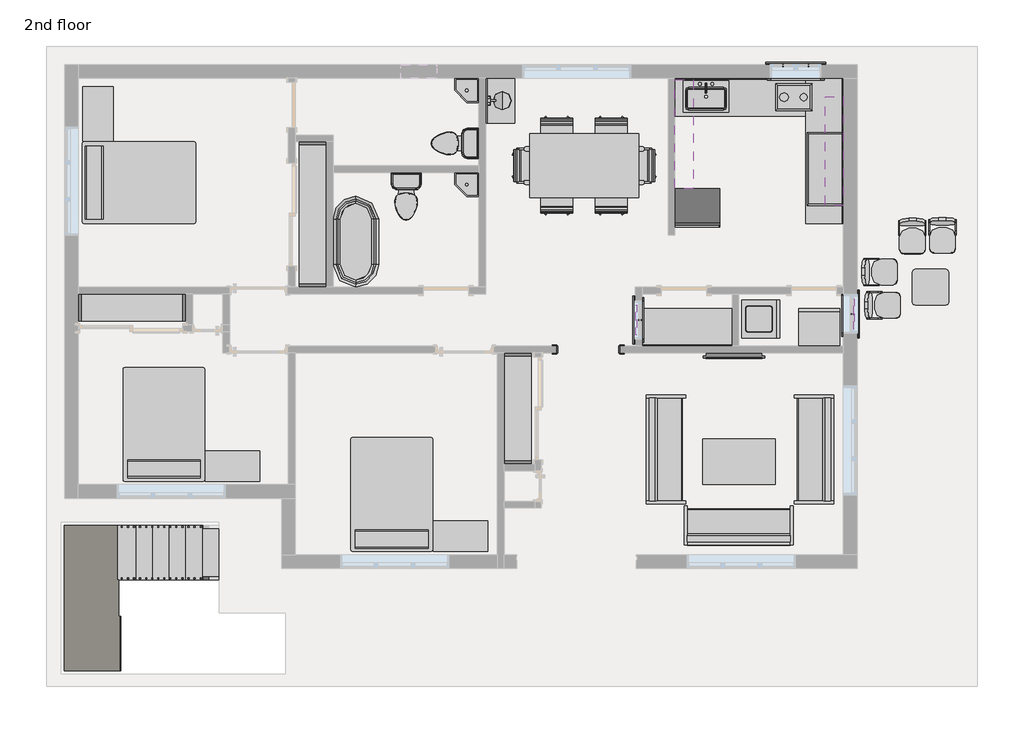
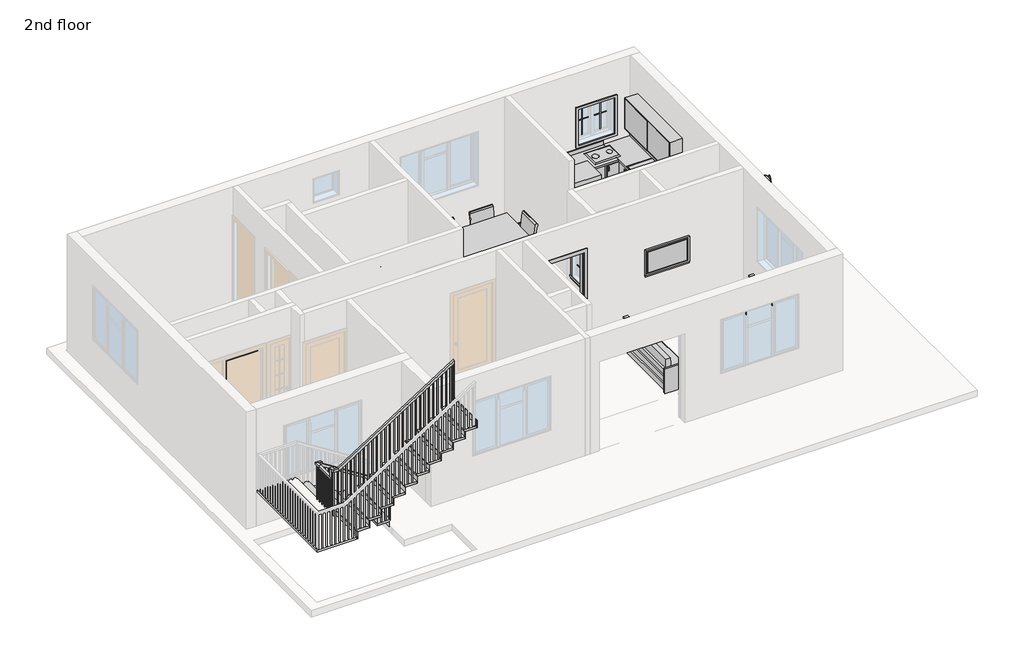
# One storey, part 4 of 4: 34 furniture elements, 17 proxies, 7 flow terminals, 2 stair flights, 1 railing, 1 slab.
"""IFC4 building model written with IfcOpenShell, lengths in millimetres."""

from ifc_helpers import new_model, si_unit, frame, origin, place, context, project, spatial, polyline, outline, extrude, faceted_brep, transform, mapped, element, save
from components import proxy_3c1fa1d0, proxy_97c73763, muntin_pattern_2x2_muntin_pattern_2x2_b3fe6957, muntin_pattern_2x2_muntin_pattern_2x2_3e0ecaf2, muntin_pattern_2x2_muntin_pattern_2x2_c35c595f, muntin_pattern_2x2_muntin_pattern_2x2_183aef24, proxy_bc9927fa, proxy_e6cf46b9, trim_window_exterior_flat_with_sill_41619996, trim_window_exterior_flat_with_sill_e38017c9, trim_window_exterior_flat_with_sill_5e960bf5, trim_window_interior_flat_picture_frame_51c85655, trim_window_interior_flat_picture_frame_d728ed12, trim_window_interior_flat_picture_frame_80babb00, proxy_1934c8a4, flow_terminal_15267b2a, flow_terminal_5b58e753, flow_terminal_4d548711, toilet_domestic_3d_toilet_domestic_3d_ba6479b0, toilet_domestic_3d_toilet_domestic_3d_30431060, flow_terminal_ce36f001, furniture_48488436, furniture_f87f75a4, furniture_97fe820d, furniture_52ef1662, furniture_6b884072, chair_task_chair_task_b7f3823b, chair_task_arms_chair_task_arms_fa5a08ef, furniture_deb1c5d1, furniture_9388d8e7, furniture_74614b7d, furniture_eb3a3c23, furniture_53a00f75, furniture_df918c0e, furniture_57be741f, furniture_57f9710a, furniture_acc2807d, furniture_65ba067b, furniture_5d68651d, furniture_b6aab1a0, furniture_1cc80a06, non_monolithic_landing_c00d822c, stair_flight_b9929406, stair_flight_87f1d909

model = new_model("IFC4")

# Units and contexts
model_context = context("Model", 3, world=origin())
ifc_project = project(units=[si_unit("LENGTHUNIT", "METRE", prefix="MILLI")], contexts=[model_context])

# Site, building, storey
site = spatial("IfcSite", under=ifc_project)
building = spatial("IfcBuilding", under=site)
storey = spatial("IfcBuildingStorey", under=building, Name="2nd floor", Elevation=7010.4)

# Proxies
placement = place(None, origin())
proxy_shape = proxy_3c1fa1d0(model_context)
element("IfcBuildingElementProxy", 1, Name="Cook Top-2 Unit : 12\" x 18\"", ObjectType="Cook Top-2 Unit : 12\" x 18\"", at=placement, inside=storey, context=model_context, shape_type="MappedRepresentation", body=[
    mapped(proxy_shape, transform((3099.7984427, 6060.3661978, 7010.4), x_axis=(0.0, 1.0, 0.0), y_axis=(-1.0, 0.0, 0.0), z_axis=(0.0, 0.0, 1.0))),
])
proxy_2_shape = proxy_97c73763(model_context)
element("IfcBuildingElementProxy", 2, Name="Dryer : 27\" x 25\" x 35\"", ObjectType="Dryer : 27\" x 25\" x 35\"", at=placement, inside=storey, context=model_context, shape_type="MappedRepresentation", body=[
    mapped(proxy_2_shape, transform((3116.0361908, 1961.105194, 7010.4), x_axis=(1.0, 0.0, 0.0), y_axis=(0.0, 1.0, 0.0), z_axis=(0.0, 0.0, 1.0))),
])
muntin_pattern_2x2_muntin_pattern_2x2_shape = muntin_pattern_2x2_muntin_pattern_2x2_b3fe6957(model_context)
element("IfcBuildingElementProxy", 3, Name="Muntin Pattern_2x2 : Muntin Pattern_2x2", ObjectType="Muntin Pattern_2x2 : Muntin Pattern_2x2", at=placement, inside=storey, context=model_context, shape_type="MappedRepresentation", body=[
    mapped(muntin_pattern_2x2_muntin_pattern_2x2_shape, transform((2887.0111471, 6673.1411978, 8172.45), x_axis=(1.0, 0.0, 0.0), y_axis=(0.0, 1.0, 0.0), z_axis=(0.0, 0.0, 1.0))),
])
muntin_pattern_2x2_muntin_pattern_2x2_2_shape = muntin_pattern_2x2_muntin_pattern_2x2_3e0ecaf2(model_context)
element("IfcBuildingElementProxy", 4, Name="Muntin Pattern_2x2 : Muntin Pattern_2x2", ObjectType="Muntin Pattern_2x2 : Muntin Pattern_2x2", at=placement, inside=storey, context=model_context, shape_type="MappedRepresentation", body=[
    mapped(muntin_pattern_2x2_muntin_pattern_2x2_2_shape, transform((3315.6361471, 6673.1411978, 8172.45), x_axis=(-1.0, 0.0, 0.0), y_axis=(0.0, -1.0, 0.0), z_axis=(0.0, 0.0, 1.0))),
])
muntin_pattern_2x2_muntin_pattern_2x2_3_shape = muntin_pattern_2x2_muntin_pattern_2x2_c35c595f(model_context)
element("IfcBuildingElementProxy", 5, Name="Muntin Pattern_2x2 : Muntin Pattern_2x2", ObjectType="Muntin Pattern_2x2 : Muntin Pattern_2x2", at=placement, inside=storey, context=model_context, shape_type="MappedRepresentation", body=[
    mapped(muntin_pattern_2x2_muntin_pattern_2x2_3_shape, transform((4095.0986471, 2498.0161978, 8480.425), x_axis=(0.0, -1.0, 0.0), y_axis=(1.0, 0.0, 0.0), z_axis=(0.0, 0.0, 1.0))),
])
element("IfcBuildingElementProxy", 6, Name="Muntin Pattern_2x2 : Muntin Pattern_2x2", ObjectType="Muntin Pattern_2x2 : Muntin Pattern_2x2", at=placement, inside=storey, context=model_context, shape_type="MappedRepresentation", body=[
    mapped(muntin_pattern_2x2_muntin_pattern_2x2_3_shape, transform((4050.6486471, 2498.0161978, 8001.0), x_axis=(0.0, -1.0, 0.0), y_axis=(1.0, 0.0, 0.0), z_axis=(0.0, 0.0, 1.0))),
])
muntin_pattern_2x2_muntin_pattern_2x2_4_shape = muntin_pattern_2x2_muntin_pattern_2x2_183aef24(model_context)
element("IfcBuildingElementProxy", 7, Name="Muntin Pattern_2x2 : Muntin Pattern_2x2", ObjectType="Muntin Pattern_2x2 : Muntin Pattern_2x2", at=placement, inside=storey, context=model_context, shape_type="MappedRepresentation", body=[
    mapped(muntin_pattern_2x2_muntin_pattern_2x2_4_shape, transform((443.8486471, 2396.4161978, 8480.425), x_axis=(0.0, -1.0, 0.0), y_axis=(1.0, 0.0, 0.0), z_axis=(0.0, 0.0, 1.0))),
])
element("IfcBuildingElementProxy", 8, Name="Muntin Pattern_2x2 : Muntin Pattern_2x2", ObjectType="Muntin Pattern_2x2 : Muntin Pattern_2x2", at=placement, inside=storey, context=model_context, shape_type="MappedRepresentation", body=[
    mapped(muntin_pattern_2x2_muntin_pattern_2x2_4_shape, transform((488.2986471, 2396.4161978, 8001.0), x_axis=(0.0, -1.0, 0.0), y_axis=(1.0, 0.0, 0.0), z_axis=(0.0, 0.0, 1.0))),
])
proxy_3_shape = proxy_bc9927fa(model_context)
element("IfcBuildingElementProxy", 9, Name="Passage Opening-Cased : 36\" x 84\"", ObjectType="Passage Opening-Cased : 36\" x 84\"", at=placement, inside=storey, context=model_context, shape_type="MappedRepresentation", body=[
    mapped(proxy_3_shape, transform((-386.6650096, 1901.1161978, 7010.4), x_axis=(-1.0, 0.0, 0.0), y_axis=(0.0, -1.0, 0.0), z_axis=(0.0, 0.0, 1.0))),
])
proxy_4_shape = proxy_e6cf46b9(model_context)
element("IfcBuildingElementProxy", 10, Name="Refrigerator-Built-in : 30\" x 24\" RH", ObjectType="Refrigerator-Built-in : 30\" x 24\" RH", at=placement, inside=storey, context=model_context, shape_type="MappedRepresentation", body=[
    mapped(proxy_4_shape, transform((1450.3236471, 4309.7422263, 7010.4), x_axis=(1.0, 0.0, 0.0), y_axis=(0.0, 1.0, 0.0), z_axis=(0.0, 0.0, 1.0))),
])
trim_window_exterior_flat_with_sill_shape = trim_window_exterior_flat_with_sill_41619996(model_context)
element("IfcBuildingElementProxy", 11, Name="Trim-Window-Exterior-Flat : with Sill", ObjectType="Trim-Window-Exterior-Flat : with Sill", at=placement, inside=storey, context=model_context, shape_type="MappedRepresentation", body=[
    mapped(trim_window_exterior_flat_with_sill_shape, transform((3101.3236471, 6682.6661978, 9017.0), x_axis=(-1.0, 0.0, 0.0), y_axis=(0.0, 0.0, 1.0), z_axis=(0.0, 1.0, 0.0))),
])
trim_window_exterior_flat_with_sill_2_shape = trim_window_exterior_flat_with_sill_e38017c9(model_context)
element("IfcBuildingElementProxy", 12, Name="Trim-Window-Exterior-Flat : with Sill", ObjectType="Trim-Window-Exterior-Flat : with Sill", at=placement, inside=storey, context=model_context, shape_type="MappedRepresentation", body=[
    mapped(trim_window_exterior_flat_with_sill_2_shape, transform((4130.0236471, 2498.0161978, 8991.6), x_axis=(0.0, 1.0, 0.0), y_axis=(0.0, 0.0, 1.0), z_axis=(1.0, 0.0, 0.0))),
])
trim_window_exterior_flat_with_sill_3_shape = trim_window_exterior_flat_with_sill_5e960bf5(model_context)
element("IfcBuildingElementProxy", 13, Name="Trim-Window-Exterior-Flat : with Sill", ObjectType="Trim-Window-Exterior-Flat : with Sill", at=placement, inside=storey, context=model_context, shape_type="MappedRepresentation", body=[
    mapped(trim_window_exterior_flat_with_sill_3_shape, transform((408.9236471, 2396.4161978, 8991.6), x_axis=(0.0, 1.0, 0.0), y_axis=(0.0, 0.0, -1.0), z_axis=(-1.0, 0.0, 0.0))),
])
trim_window_interior_flat_picture_frame_shape = trim_window_interior_flat_picture_frame_51c85655(model_context)
element("IfcBuildingElementProxy", 14, Name="Trim-Window-Interior-Flat : Picture Frame", ObjectType="Trim-Window-Interior-Flat : Picture Frame", at=placement, inside=storey, context=model_context, shape_type="MappedRepresentation", body=[
    mapped(trim_window_interior_flat_picture_frame_shape, transform((3101.3236471, 6454.0661978, 9017.0), x_axis=(1.0, 0.0, 0.0), y_axis=(0.0, 0.0, 1.0), z_axis=(0.0, -1.0, 0.0))),
])
trim_window_interior_flat_picture_frame_2_shape = trim_window_interior_flat_picture_frame_d728ed12(model_context)
element("IfcBuildingElementProxy", 15, Name="Trim-Window-Interior-Flat : Picture Frame", ObjectType="Trim-Window-Interior-Flat : Picture Frame", at=placement, inside=storey, context=model_context, shape_type="MappedRepresentation", body=[
    mapped(trim_window_interior_flat_picture_frame_2_shape, transform((3901.4236471, 2498.0161978, 8991.6), x_axis=(0.0, -1.0, 0.0), y_axis=(0.0, 0.0, 1.0), z_axis=(-1.0, 0.0, 0.0))),
])
trim_window_interior_flat_picture_frame_3_shape = trim_window_interior_flat_picture_frame_80babb00(model_context)
element("IfcBuildingElementProxy", 16, Name="Trim-Window-Interior-Flat : Picture Frame", ObjectType="Trim-Window-Interior-Flat : Picture Frame", at=placement, inside=storey, context=model_context, shape_type="MappedRepresentation", body=[
    mapped(trim_window_interior_flat_picture_frame_3_shape, transform((523.2236471, 2396.4161978, 8991.6), x_axis=(0.0, -1.0, 0.0), y_axis=(0.0, 0.0, -1.0), z_axis=(1.0, 0.0, 0.0))),
])
proxy_5_shape = proxy_1934c8a4(model_context)
element("IfcBuildingElementProxy", 17, Name="Washer : 25\" x 25\" x 35\"", ObjectType="Washer : 25\" x 25\" x 35\"", at=placement, inside=storey, context=model_context, shape_type="MappedRepresentation", body=[
    mapped(proxy_5_shape, transform((2237.9740823, 2809.1661978, 7010.4), x_axis=(0.0, -1.0, 0.0), y_axis=(1.0, 0.0, 0.0), z_axis=(0.0, 0.0, 1.0))),
])

# Flow terminals
flow_terminal_shape = flow_terminal_15267b2a(model_context)
element("IfcFlowTerminal", 18, ObjectType="Lavatory - Vanity : 30\"x18\" - Private", at=placement, inside=storey, context=model_context, shape_type="MappedRepresentation", body=[
    mapped(flow_terminal_shape, transform((-2099.3263529, 6079.4161978, 7010.4), x_axis=(1.0, 0.0, 0.0), y_axis=(0.0, 1.0, 0.0), z_axis=(0.0, 0.0, 1.0))),
])
flow_terminal_2_shape = flow_terminal_5b58e753(model_context)
element("IfcFlowTerminal", 19, ObjectType="Sink - Mop : 28\"x28\"", at=placement, inside=storey, context=model_context, shape_type="MappedRepresentation", body=[
    mapped(flow_terminal_2_shape, transform((-2213.6263529, 4872.9161978, 7010.4), x_axis=(0.0, -1.0, 0.0), y_axis=(1.0, 0.0, 0.0), z_axis=(0.0, 0.0, 1.0))),
])
element("IfcFlowTerminal", 20, ObjectType="Sink - Mop : 28\"x28\"", at=placement, inside=storey, context=model_context, shape_type="MappedRepresentation", body=[
    mapped(flow_terminal_2_shape, transform((-2213.6263529, 6454.0661978, 7010.4), x_axis=(0.0, -1.0, 0.0), y_axis=(1.0, 0.0, 0.0), z_axis=(0.0, 0.0, 1.0))),
])
flow_terminal_3_shape = flow_terminal_4d548711(model_context)
element("IfcFlowTerminal", 21, ObjectType="Sink Kitchen-Single : 30\" x 21\"", at=placement, inside=storey, context=model_context, shape_type="MappedRepresentation", body=[
    mapped(flow_terminal_3_shape, transform((1580.6844065, 6146.9207967, 7010.4), x_axis=(1.0, 0.0, 0.0), y_axis=(0.0, 1.0, 0.0), z_axis=(0.0, 0.0, 1.0))),
])
toilet_domestic_3d_toilet_domestic_3d_shape = toilet_domestic_3d_toilet_domestic_3d_ba6479b0(model_context)
toilet_domestic_3d_toilet_domestic_3d_2_shape = toilet_domestic_3d_toilet_domestic_3d_30431060(model_context)
element("IfcFlowTerminal", 22, ObjectType="Toilet-Domestic-3D : Toilet-Domestic-3D", at=placement, inside=storey, context=model_context, shape_type="MappedRepresentation", body=[
    mapped(toilet_domestic_3d_toilet_domestic_3d_shape, transform((-3433.7493286, 4378.2201704, 7010.4), x_axis=(1.0, 0.0, 0.0), y_axis=(0.0, 1.0, 0.0), z_axis=(0.0, 0.0, 1.0))),
    mapped(toilet_domestic_3d_toilet_domestic_3d_2_shape, transform((-3433.7493286, 4378.2201704, 7010.4), x_axis=(1.0, 0.0, 0.0), y_axis=(0.0, 1.0, 0.0), z_axis=(0.0, 0.0, 1.0))),
])
element("IfcFlowTerminal", 23, ObjectType="Toilet-Domestic-3D : Toilet-Domestic-3D", at=placement, inside=storey, context=model_context, shape_type="MappedRepresentation", body=[
    mapped(toilet_domestic_3d_toilet_domestic_3d_shape, transform((-2708.3223803, 5361.8661978, 7010.4), x_axis=(0.0, -1.0, 0.0), y_axis=(1.0, 0.0, 0.0), z_axis=(0.0, 0.0, 1.0))),
    mapped(toilet_domestic_3d_toilet_domestic_3d_2_shape, transform((-2708.3223803, 5361.8661978, 7010.4), x_axis=(0.0, -1.0, 0.0), y_axis=(1.0, 0.0, 0.0), z_axis=(0.0, 0.0, 1.0))),
])
flow_terminal_4_shape = flow_terminal_ce36f001(model_context)
element("IfcFlowTerminal", 24, ObjectType="Tub-Free Standing-3D : 30\" x 60\"", at=placement, inside=storey, context=model_context, shape_type="MappedRepresentation", body=[
    mapped(flow_terminal_4_shape, transform((-4277.3763529, 3710.8661978, 7010.4), x_axis=(-1.0, 0.0, 0.0), y_axis=(0.0, -1.0, 0.0), z_axis=(0.0, 0.0, 1.0))),
])

# Furniture
furniture_shape = furniture_48488436(model_context)
element("IfcFurniture", 25, ObjectType="48\"", at=placement, inside=storey, context=model_context, shape_type="MappedRepresentation", body=[
    mapped(furniture_shape, transform((3901.4236471, 5020.9111578, 7010.4), x_axis=(0.0, -1.0, 0.0), y_axis=(1.0, 0.0, 0.0), z_axis=(0.0, 0.0, 1.0))),
])
furniture_2_shape = furniture_f87f75a4(model_context)
element("IfcFurniture", 26, ObjectType="Base Cabinet-Combo01 : 30\"", at=placement, inside=storey, context=model_context, shape_type="MappedRepresentation", body=[
    mapped(furniture_2_shape, transform((2587.2859422, 6454.0661978, 7010.4), x_axis=(1.0, 0.0, 0.0), y_axis=(0.0, 1.0, 0.0), z_axis=(0.0, 0.0, 1.0))),
])
furniture_3_shape = furniture_97fe820d(model_context)
element("IfcFurniture", 27, ObjectType="Base Cabinet-Corner Unit-Square : 36\"", at=placement, inside=storey, context=model_context, shape_type="MappedRepresentation", body=[
    mapped(furniture_3_shape, transform((3374.6859422, 6454.0661978, 7010.4), x_axis=(1.0, 0.0, 0.0), y_axis=(0.0, 1.0, 0.0), z_axis=(0.0, 0.0, 1.0))),
])
furniture_4_shape = furniture_52ef1662(model_context)
element("IfcFurniture", 28, ObjectType="Bed-Standard : Double 54\" x 75\"", at=placement, inside=storey, context=model_context, shape_type="MappedRepresentation", body=[
    mapped(furniture_4_shape, transform((-7961.5214349, 4429.9776732, 7010.4), x_axis=(0.0, 1.0, 0.0), y_axis=(-1.0, 0.0, 0.0), z_axis=(0.0, 0.0, 1.0))),
])
element("IfcFurniture", 29, ObjectType="Bed-Standard : Double 54\" x 75\"", at=placement, inside=storey, context=model_context, shape_type="MappedRepresentation", body=[
    mapped(furniture_4_shape, transform((-7225.3378283, 598.2211158, 7010.4), x_axis=(-1.0, 0.0, 0.0), y_axis=(0.0, -1.0, 0.0), z_axis=(0.0, 0.0, 1.0))),
])
element("IfcFurniture", 30, ObjectType="Bed-Standard : Double 54\" x 75\"", at=placement, inside=storey, context=model_context, shape_type="MappedRepresentation", body=[
    mapped(furniture_4_shape, transform((-3402.6378283, -576.5288842, 7010.4), x_axis=(-1.0, 0.0, 0.0), y_axis=(0.0, -1.0, 0.0), z_axis=(0.0, 0.0, 1.0))),
])
furniture_5_shape = furniture_6b884072(model_context)
element("IfcFurniture", 31, ObjectType="Cabinet File-Lateral 2 Drawer : 36\" x 20\" x 24\"", at=placement, inside=storey, context=model_context, shape_type="MappedRepresentation", body=[
    mapped(furniture_5_shape, transform((-9536.044729, 6037.1887117, 7010.4), x_axis=(0.0, 1.0, 0.0), y_axis=(-1.0, 0.0, 0.0), z_axis=(0.0, 0.0, 1.0))),
])
element("IfcFurniture", 32, ObjectType="Cabinet File-Lateral 2 Drawer : 36\" x 20\" x 24\"", at=placement, inside=storey, context=model_context, shape_type="MappedRepresentation", body=[
    mapped(furniture_5_shape, transform((-6527.4988668, -989.0021783, 7010.4), x_axis=(-1.0, 0.0, 0.0), y_axis=(0.0, -1.0, 0.0), z_axis=(0.0, 0.0, 1.0))),
])
element("IfcFurniture", 33, ObjectType="Cabinet File-Lateral 2 Drawer : 36\" x 20\" x 24\"", at=placement, inside=storey, context=model_context, shape_type="MappedRepresentation", body=[
    mapped(furniture_5_shape, transform((-2698.4488668, -2163.7521783, 7010.4), x_axis=(-1.0, 0.0, 0.0), y_axis=(0.0, -1.0, 0.0), z_axis=(0.0, 0.0, 1.0))),
])
chair_task_chair_task_shape = chair_task_chair_task_b7f3823b(model_context)
element("IfcFurniture", 34, ObjectType="Chair-Task : Chair-Task", at=placement, inside=storey, context=model_context, shape_type="MappedRepresentation", body=[
    mapped(chair_task_chair_task_shape, transform((149.8644668, 5539.5620994, 7010.4), x_axis=(-1.0, 0.0, 0.0), y_axis=(0.0, -1.0, 0.0), z_axis=(0.0, 0.0, 1.0))),
])
element("IfcFurniture", 35, ObjectType="Chair-Task : Chair-Task", at=placement, inside=storey, context=model_context, shape_type="MappedRepresentation", body=[
    mapped(chair_task_chair_task_shape, transform((-132.1171726, 4434.8702962, 7010.4), x_axis=(1.0, 0.0, 0.0), y_axis=(0.0, 1.0, 0.0), z_axis=(0.0, 0.0, 1.0))),
])
element("IfcFurniture", 36, ObjectType="Chair-Task : Chair-Task", at=placement, inside=storey, context=model_context, shape_type="MappedRepresentation", body=[
    mapped(chair_task_chair_task_shape, transform((-764.5355332, 5539.5620994, 7010.4), x_axis=(-1.0, 0.0, 0.0), y_axis=(0.0, -1.0, 0.0), z_axis=(0.0, 0.0, 1.0))),
])
element("IfcFurniture", 37, ObjectType="Chair-Task : Chair-Task", at=placement, inside=storey, context=model_context, shape_type="MappedRepresentation", body=[
    mapped(chair_task_chair_task_shape, transform((-1046.5171726, 4434.8702962, 7010.4), x_axis=(1.0, 0.0, 0.0), y_axis=(0.0, 1.0, 0.0), z_axis=(0.0, 0.0, 1.0))),
])
chair_task_arms_chair_task_arms_shape = chair_task_arms_chair_task_arms_fa5a08ef(model_context)
element("IfcFurniture", 38, ObjectType="Chair-Task Arms : Chair-Task Arms", at=placement, inside=storey, context=model_context, shape_type="MappedRepresentation", body=[
    mapped(chair_task_arms_chair_task_arms_shape, transform((-1381.6722545, 5128.2070175, 7010.4), x_axis=(0.0, -1.0, 0.0), y_axis=(1.0, 0.0, 0.0), z_axis=(0.0, 0.0, 1.0))),
])
element("IfcFurniture", 39, ObjectType="Chair-Task Arms : Chair-Task Arms", at=placement, inside=storey, context=model_context, shape_type="MappedRepresentation", body=[
    mapped(chair_task_arms_chair_task_arms_shape, transform((485.0195487, 4846.2253781, 7010.4), x_axis=(0.0, 1.0, 0.0), y_axis=(-1.0, 0.0, 0.0), z_axis=(0.0, 0.0, 1.0))),
])
furniture_6_shape = furniture_deb1c5d1(model_context)
element("IfcFurniture", 40, ObjectType="Counter Top : 24\" Depth", at=placement, inside=storey, context=model_context, shape_type="MappedRepresentation", body=[
    mapped(furniture_6_shape, transform((3901.4236471, 5253.6039027, 7010.4), x_axis=(0.0, -1.0, 0.0), y_axis=(1.0, 0.0, 0.0), z_axis=(0.0, 0.0, 1.0))),
])
furniture_7_shape = furniture_9388d8e7(model_context)
element("IfcFurniture", 41, ObjectType="Counter Top : 24\" Depth", at=placement, inside=storey, context=model_context, shape_type="MappedRepresentation", body=[
    mapped(furniture_7_shape, transform((834.061352, 1958.2661978, 7010.4), x_axis=(-1.0, 0.0, 0.0), y_axis=(0.0, -1.0, 0.0), z_axis=(0.0, 0.0, 1.0))),
])
furniture_8_shape = furniture_74614b7d(model_context)
element("IfcFurniture", 42, ObjectType="Counter Top w Sink Hole : 24\" Depth", at=placement, inside=storey, context=model_context, shape_type="MappedRepresentation", body=[
    mapped(furniture_8_shape, transform((2276.1359422, 6454.0661978, 7010.4), x_axis=(1.0, 0.0, 0.0), y_axis=(0.0, 1.0, 0.0), z_axis=(0.0, 0.0, 1.0))),
])
furniture_9_shape = furniture_eb3a3c23(model_context)
element("IfcFurniture", 43, ObjectType="Seating-Auditorium : 18\" x 24\" x 30\"", at=placement, inside=storey, context=model_context, shape_type="MappedRepresentation", body=[
    mapped(furniture_9_shape, transform((4308.4482373, 3363.5940666, 7010.4), x_axis=(0.0, -1.0, 0.0), y_axis=(1.0, 0.0, 0.0), z_axis=(0.0, 0.0, 1.0))),
])
element("IfcFurniture", 44, ObjectType="Seating-Auditorium : 18\" x 24\" x 30\"", at=placement, inside=storey, context=model_context, shape_type="MappedRepresentation", body=[
    mapped(furniture_9_shape, transform((4359.2482373, 2804.7940666, 7010.4), x_axis=(0.0, -1.0, 0.0), y_axis=(1.0, 0.0, 0.0), z_axis=(0.0, 0.0, 1.0))),
])
element("IfcFurniture", 45, ObjectType="Seating-Auditorium : 18\" x 24\" x 30\"", at=placement, inside=storey, context=model_context, shape_type="MappedRepresentation", body=[
    mapped(furniture_9_shape, transform((5217.8515159, 4002.3416076, 7010.4), x_axis=(-1.0, 0.0, 0.0), y_axis=(0.0, -1.0, 0.0), z_axis=(0.0, 0.0, 1.0))),
])
element("IfcFurniture", 46, ObjectType="Seating-Auditorium : 18\" x 24\" x 30\"", at=placement, inside=storey, context=model_context, shape_type="MappedRepresentation", body=[
    mapped(furniture_9_shape, transform((5725.8515159, 4015.0416076, 7010.4), x_axis=(-1.0, 0.0, 0.0), y_axis=(0.0, -1.0, 0.0), z_axis=(0.0, 0.0, 1.0))),
])
furniture_10_shape = furniture_53a00f75(model_context)
element("IfcFurniture", 47, ObjectType="Shelving : 96\" x 12\" x 84\"", at=placement, inside=storey, context=model_context, shape_type="MappedRepresentation", body=[
    mapped(furniture_10_shape, transform((-1864.3763529, 910.5161978, 7010.4), x_axis=(0.0, 1.0, 0.0), y_axis=(-1.0, 0.0, 0.0), z_axis=(0.0, 0.0, 1.0))),
])
furniture_11_shape = furniture_df918c0e(model_context)
element("IfcFurniture", 48, ObjectType="Shelving : 96\" x 12\" x 84\" 2", at=placement, inside=storey, context=model_context, shape_type="MappedRepresentation", body=[
    mapped(furniture_11_shape, transform((-8030.2263529, 2910.7661978, 7010.4), x_axis=(1.0, 0.0, 0.0), y_axis=(0.0, 1.0, 0.0), z_axis=(0.0, 0.0, 1.0))),
])
furniture_12_shape = furniture_57be741f(model_context)
element("IfcFurniture", 49, ObjectType="Shelving : 96\" x 12\" x 84\" 3", at=placement, inside=storey, context=model_context, shape_type="MappedRepresentation", body=[
    mapped(furniture_12_shape, transform((-5306.0763529, 4168.0661978, 7010.4), x_axis=(0.0, 1.0, 0.0), y_axis=(-1.0, 0.0, 0.0), z_axis=(0.0, 0.0, 1.0))),
])
furniture_13_shape = furniture_57f9710a(model_context)
element("IfcFurniture", 50, ObjectType="Sofa : 72\"", at=placement, inside=storey, context=model_context, shape_type="MappedRepresentation", body=[
    mapped(furniture_13_shape, transform((2219.1941389, -905.4797038, 7010.4), x_axis=(-1.0, 0.0, 0.0), y_axis=(0.0, -1.0, 0.0), z_axis=(0.0, 0.0, 1.0))),
])
element("IfcFurniture", 51, ObjectType="Sofa : 72\"", at=placement, inside=storey, context=model_context, shape_type="MappedRepresentation", body=[
    mapped(furniture_13_shape, transform((3259.9695487, 295.0866896, 7010.4), x_axis=(0.0, -1.0, 0.0), y_axis=(1.0, 0.0, 0.0), z_axis=(0.0, 0.0, 1.0))),
])
element("IfcFurniture", 52, ObjectType="Sofa : 72\"", at=placement, inside=storey, context=model_context, shape_type="MappedRepresentation", body=[
    mapped(furniture_13_shape, transform((1069.4277455, 154.345706, 7010.4), x_axis=(0.0, 1.0, 0.0), y_axis=(-1.0, 0.0, 0.0), z_axis=(0.0, 0.0, 1.0))),
])
furniture_14_shape = furniture_acc2807d(model_context)
element("IfcFurniture", 53, ObjectType="Table-Coffee Rectangular : 48\" x 30\"", at=placement, inside=storey, context=model_context, shape_type="MappedRepresentation", body=[
    mapped(furniture_14_shape, transform((1535.4900168, -354.444634, 7010.4), x_axis=(1.0, 0.0, 0.0), y_axis=(0.0, 1.0, 0.0), z_axis=(0.0, 0.0, 1.0))),
])
furniture_15_shape = furniture_65ba067b(model_context)
element("IfcFurniture", 54, ObjectType="Table-Conference2 w Chairs : 40\" x 90\"", at=placement, inside=storey, context=model_context, shape_type="MappedRepresentation", body=[
    mapped(furniture_15_shape, transform((-448.3263529, 4987.2161978, 7010.4), x_axis=(1.0, 0.0, 0.0), y_axis=(0.0, 1.0, 0.0), z_axis=(0.0, 0.0, 1.0))),
])
furniture_16_shape = furniture_5d68651d(model_context)
element("IfcFurniture", 55, ObjectType="Table-End : 24\" x 24\"", at=placement, inside=storey, context=model_context, shape_type="MappedRepresentation", body=[
    mapped(furniture_16_shape, transform((5053.3900168, 2796.4661978, 7010.4), x_axis=(1.0, 0.0, 0.0), y_axis=(0.0, 1.0, 0.0), z_axis=(0.0, 0.0, 1.0))),
])
furniture_17_shape = furniture_b6aab1a0(model_context)
element("IfcFurniture", 56, ObjectType="Television-Plasma : 42\"", at=placement, inside=storey, context=model_context, shape_type="MappedRepresentation", body=[
    mapped(furniture_17_shape, transform((2009.1236471, 1843.9661978, 8077.2), x_axis=(1.0, 0.0, 0.0), y_axis=(0.0, 1.0, 0.0), z_axis=(0.0, 0.0, 1.0))),
])
furniture_18_shape = furniture_1cc80a06(model_context)
element("IfcFurniture", 57, ObjectType="Upper Cabinet-Pass-Thru w Glass : 48\" x 30\" x 12\"", at=placement, inside=storey, context=model_context, shape_type="MappedRepresentation", body=[
    mapped(furniture_18_shape, transform((1075.6736471, 5495.5284929, 7010.4), x_axis=(0.0, 1.0, 0.0), y_axis=(-1.0, 0.0, 0.0), z_axis=(0.0, 0.0, 1.0))),
])
element("IfcFurniture", 58, ObjectType="Upper Cabinet-Pass-Thru w Glass : 48\" x 30\" x 12\"", at=placement, inside=storey, context=model_context, shape_type="MappedRepresentation", body=[
    mapped(furniture_18_shape, transform((3596.6236471, 5216.1284929, 7010.4), x_axis=(0.0, 1.0, 0.0), y_axis=(-1.0, 0.0, 0.0), z_axis=(0.0, 0.0, 1.0))),
])

# Railing
element("IfcRailing", 59, ObjectType="Handrail - Rectangular", at=placement, inside=storey, context=model_context, shape_type="SolidModel", body=[
    faceted_brep([(-6576.0763529, -1966.0338022, 8102.6), (-6576.0763529, -1966.0338022, 8042.386276), (-6576.0763529, -1915.2338022, 8042.386276), (-6576.0763529, -1915.2338022, 8102.6), (-8176.2763529, -1966.0338022, 9120.9090909), (-8227.0763529, -1966.0338022, 9093.0226396), (-8227.0763529, -1915.2338022, 9093.0226396), (-8176.2763529, -1915.2338022, 9120.9090909), (-8176.2763529, -1966.0338022, 9169.4), (-8227.0763529, -1966.0338022, 9118.6), (-8227.0763529, -1915.2338022, 9118.6), (-8176.2763529, -1915.2338022, 9169.4), (-8252.4763529, -1966.0338022, 9169.4), (-8252.4763529, -1966.0338022, 9118.6), (-8303.2763529, -1915.2338022, 9118.6), (-8303.2763529, -1915.2338022, 9169.4), (-8252.4763529, -2042.2338022, 9169.4), (-8252.4763529, -2042.2338022, 9118.6), (-8303.2763529, -2042.2338022, 9118.6), (-8303.2763529, -2042.2338022, 9169.4), (-8252.4763529, -2499.4338022, 9169.4), (-8252.4763529, -2550.2338022, 9118.6), (-8303.2763529, -2550.2338022, 9118.6), (-8303.2763529, -2499.4338022, 9169.4), (-8252.4763529, -2499.4338022, 9395.6909091), (-8252.4763529, -2550.2338022, 9344.8909091), (-8303.2763529, -2550.2338022, 9344.8909091), (-8303.2763529, -2499.4338022, 9395.6909091), (-8252.4763529, -2575.6338022, 9395.6909091), (-8252.4763529, -2575.6338022, 9344.8909091), (-8303.2763529, -2626.4338022, 9344.8909091), (-8303.2763529, -2626.4338022, 9395.6909091), (-8176.2763529, -2575.6338022, 9395.6909091), (-8161.483358, -2575.6338022, 9344.8909091), (-8161.483358, -2626.4338022, 9344.8909091), (-8176.2763529, -2626.4338022, 9395.6909091), (-5458.4763529, -2575.6338022, 11125.2), (-5458.4763529, -2626.4338022, 11125.2), (-5458.4763529, -2626.4338022, 11064.986276), (-5458.4763529, -2575.6338022, 11064.986276)], [[[0, 1, 2, 3]], [[1, 0, 4, 5]], [[2, 1, 5, 6]], [[3, 2, 6, 7]], [[0, 3, 7, 4]], [[5, 4, 8, 9]], [[6, 5, 9, 10]], [[7, 6, 10, 11]], [[4, 7, 11, 8]], [[9, 8, 12, 13]], [[10, 9, 13, 14]], [[11, 10, 14, 15]], [[8, 11, 15, 12]], [[13, 12, 16, 17]], [[14, 13, 17, 18]], [[15, 14, 18, 19]], [[12, 15, 19, 16]], [[17, 16, 20, 21]], [[18, 17, 21, 22]], [[19, 18, 22, 23]], [[16, 19, 23, 20]], [[21, 20, 24, 25]], [[22, 21, 25, 26]], [[23, 22, 26, 27]], [[20, 23, 27, 24]], [[25, 24, 28, 29]], [[26, 25, 29, 30]], [[27, 26, 30, 31]], [[24, 27, 31, 28]], [[29, 28, 32, 33]], [[30, 29, 33, 34]], [[31, 30, 34, 35]], [[28, 31, 35, 32]], [[36, 37, 38, 39]], [[33, 32, 36, 39]], [[34, 33, 39, 38]], [[35, 34, 38, 37]], [[32, 35, 37, 36]]]),
    extrude(outline(polyline([(11010.4340032, -5544.2013529), (10033.0, -5544.2013529), (10033.0, -5525.1513529), (11022.5567305, -5525.1513529), (11010.4340032, -5544.2013529)])), frame((0.0, -2610.5588022, 0.0), z_axis=(0.0, 1.0, 0.0), x_axis=(0.0, 0.0, 1.0)), (0.0, 0.0, 1.0), 19.05),
    extrude(outline(polyline([(10945.7794578, -5645.8013529), (10033.0, -5645.8013529), (10033.0, -5626.7513529), (10957.9021851, -5626.7513529), (10945.7794578, -5645.8013529)])), frame((0.0, -2610.5588022, 0.0), z_axis=(0.0, 1.0, 0.0), x_axis=(0.0, 0.0, 1.0)), (0.0, 0.0, 1.0), 19.05),
    extrude(outline(polyline([(10881.1249123, -5747.4013529), (10033.0, -5747.4013529), (10033.0, -5728.3513529), (10893.2476396, -5728.3513529), (10881.1249123, -5747.4013529)])), frame((0.0, -2610.5588022, 0.0), z_axis=(0.0, 1.0, 0.0), x_axis=(0.0, 0.0, 1.0)), (0.0, 0.0, 1.0), 19.05),
    extrude(outline(polyline([(10816.4703669, -5849.0013529), (9855.2, -5849.0013529), (9855.2, -5829.9513529), (10828.5930941, -5829.9513529), (10816.4703669, -5849.0013529)])), frame((0.0, -2610.5588022, 0.0), z_axis=(0.0, 1.0, 0.0), x_axis=(0.0, 0.0, 1.0)), (0.0, 0.0, 1.0), 19.05),
    extrude(outline(polyline([(10751.8158214, -5950.6013529), (9855.2, -5950.6013529), (9855.2, -5931.5513529), (10763.9385487, -5931.5513529), (10751.8158214, -5950.6013529)])), frame((0.0, -2610.5588022, 0.0), z_axis=(0.0, 1.0, 0.0), x_axis=(0.0, 0.0, 1.0)), (0.0, 0.0, 1.0), 19.05),
    extrude(outline(polyline([(10687.161276, -6052.2013529), (9677.4, -6052.2013529), (9677.4, -6033.1513529), (10699.2840032, -6033.1513529), (10687.161276, -6052.2013529)])), frame((0.0, -2610.5588022, 0.0), z_axis=(0.0, 1.0, 0.0), x_axis=(0.0, 0.0, 1.0)), (0.0, 0.0, 1.0), 19.05),
    extrude(outline(polyline([(10622.5067305, -6153.8013529), (9677.4, -6153.8013529), (9677.4, -6134.7513529), (10634.6294578, -6134.7513529), (10622.5067305, -6153.8013529)])), frame((0.0, -2610.5588022, 0.0), z_axis=(0.0, 1.0, 0.0), x_axis=(0.0, 0.0, 1.0)), (0.0, 0.0, 1.0), 19.05),
    extrude(outline(polyline([(10557.8521851, -6255.4013529), (9677.4, -6255.4013529), (9677.4, -6236.3513529), (10569.9749123, -6236.3513529), (10557.8521851, -6255.4013529)])), frame((0.0, -2610.5588022, 0.0), z_axis=(0.0, 1.0, 0.0), x_axis=(0.0, 0.0, 1.0)), (0.0, 0.0, 1.0), 19.05),
    extrude(outline(polyline([(10493.1976396, -6357.0013529), (9499.6, -6357.0013529), (9499.6, -6337.9513529), (10505.3203669, -6337.9513529), (10493.1976396, -6357.0013529)])), frame((0.0, -2610.5588022, 0.0), z_axis=(0.0, 1.0, 0.0), x_axis=(0.0, 0.0, 1.0)), (0.0, 0.0, 1.0), 19.05),
    extrude(outline(polyline([(10428.5430941, -6458.6013529), (9499.6, -6458.6013529), (9499.6, -6439.5513529), (10440.6658214, -6439.5513529), (10428.5430941, -6458.6013529)])), frame((0.0, -2610.5588022, 0.0), z_axis=(0.0, 1.0, 0.0), x_axis=(0.0, 0.0, 1.0)), (0.0, 0.0, 1.0), 19.05),
    extrude(outline(polyline([(10363.8885487, -6560.2013529), (9499.6, -6560.2013529), (9499.6, -6541.1513529), (10376.011276, -6541.1513529), (10363.8885487, -6560.2013529)])), frame((0.0, -2610.5588022, 0.0), z_axis=(0.0, 1.0, 0.0), x_axis=(0.0, 0.0, 1.0)), (0.0, 0.0, 1.0), 19.05),
    extrude(outline(polyline([(10299.2340032, -6661.8013529), (9321.8, -6661.8013529), (9321.8, -6642.7513529), (10311.3567305, -6642.7513529), (10299.2340032, -6661.8013529)])), frame((0.0, -2610.5588022, 0.0), z_axis=(0.0, 1.0, 0.0), x_axis=(0.0, 0.0, 1.0)), (0.0, 0.0, 1.0), 19.05),
    extrude(outline(polyline([(10234.5794578, -6763.4013529), (9321.8, -6763.4013529), (9321.8, -6744.3513529), (10246.7021851, -6744.3513529), (10234.5794578, -6763.4013529)])), frame((0.0, -2610.5588022, 0.0), z_axis=(0.0, 1.0, 0.0), x_axis=(0.0, 0.0, 1.0)), (0.0, 0.0, 1.0), 19.05),
    extrude(outline(polyline([(10169.9249123, -6865.0013529), (9321.8, -6865.0013529), (9321.8, -6845.9513529), (10182.0476396, -6845.9513529), (10169.9249123, -6865.0013529)])), frame((0.0, -2610.5588022, 0.0), z_axis=(0.0, 1.0, 0.0), x_axis=(0.0, 0.0, 1.0)), (0.0, 0.0, 1.0), 19.05),
    extrude(outline(polyline([(10105.2703669, -6966.6013529), (9144.0, -6966.6013529), (9144.0, -6947.5513529), (10117.3930941, -6947.5513529), (10105.2703669, -6966.6013529)])), frame((0.0, -2610.5588022, 0.0), z_axis=(0.0, 1.0, 0.0), x_axis=(0.0, 0.0, 1.0)), (0.0, 0.0, 1.0), 19.05),
    extrude(outline(polyline([(10040.6158214, -7068.2013529), (9144.0, -7068.2013529), (9144.0, -7049.1513529), (10052.7385487, -7049.1513529), (10040.6158214, -7068.2013529)])), frame((0.0, -2610.5588022, 0.0), z_axis=(0.0, 1.0, 0.0), x_axis=(0.0, 0.0, 1.0)), (0.0, 0.0, 1.0), 19.05),
    extrude(outline(polyline([(9975.961276, -7169.8013529), (8966.2, -7169.8013529), (8966.2, -7150.7513529), (9988.0840032, -7150.7513529), (9975.961276, -7169.8013529)])), frame((0.0, -2610.5588022, 0.0), z_axis=(0.0, 1.0, 0.0), x_axis=(0.0, 0.0, 1.0)), (0.0, 0.0, 1.0), 19.05),
    extrude(outline(polyline([(9911.3067305, -7271.4013529), (8966.2, -7271.4013529), (8966.2, -7252.3513529), (9923.4294578, -7252.3513529), (9911.3067305, -7271.4013529)])), frame((0.0, -2610.5588022, 0.0), z_axis=(0.0, 1.0, 0.0), x_axis=(0.0, 0.0, 1.0)), (0.0, 0.0, 1.0), 19.05),
    extrude(outline(polyline([(9846.6521851, -7373.0013529), (8966.2, -7373.0013529), (8966.2, -7353.9513529), (9858.7749123, -7353.9513529), (9846.6521851, -7373.0013529)])), frame((0.0, -2610.5588022, 0.0), z_axis=(0.0, 1.0, 0.0), x_axis=(0.0, 0.0, 1.0)), (0.0, 0.0, 1.0), 19.05),
    extrude(outline(polyline([(9781.9976396, -7474.6013529), (8788.4, -7474.6013529), (8788.4, -7455.5513529), (9794.1203669, -7455.5513529), (9781.9976396, -7474.6013529)])), frame((0.0, -2610.5588022, 0.0), z_axis=(0.0, 1.0, 0.0), x_axis=(0.0, 0.0, 1.0)), (0.0, 0.0, 1.0), 19.05),
    extrude(outline(polyline([(9717.3430941, -7576.2013529), (8788.4, -7576.2013529), (8788.4, -7557.1513529), (9729.4658214, -7557.1513529), (9717.3430941, -7576.2013529)])), frame((0.0, -2610.5588022, 0.0), z_axis=(0.0, 1.0, 0.0), x_axis=(0.0, 0.0, 1.0)), (0.0, 0.0, 1.0), 19.05),
    extrude(outline(polyline([(9652.6885487, -7677.8013529), (8788.4, -7677.8013529), (8788.4, -7658.7513529), (9664.811276, -7658.7513529), (9652.6885487, -7677.8013529)])), frame((0.0, -2610.5588022, 0.0), z_axis=(0.0, 1.0, 0.0), x_axis=(0.0, 0.0, 1.0)), (0.0, 0.0, 1.0), 19.05),
    extrude(outline(polyline([(9588.0340032, -7779.4013529), (8610.6, -7779.4013529), (8610.6, -7760.3513529), (9600.1567305, -7760.3513529), (9588.0340032, -7779.4013529)])), frame((0.0, -2610.5588022, 0.0), z_axis=(0.0, 1.0, 0.0), x_axis=(0.0, 0.0, 1.0)), (0.0, 0.0, 1.0), 19.05),
    extrude(outline(polyline([(9523.3794578, -7881.0013529), (8610.6, -7881.0013529), (8610.6, -7861.9513529), (9535.5021851, -7861.9513529), (9523.3794578, -7881.0013529)])), frame((0.0, -2610.5588022, 0.0), z_axis=(0.0, 1.0, 0.0), x_axis=(0.0, 0.0, 1.0)), (0.0, 0.0, 1.0), 19.05),
    extrude(outline(polyline([(9458.7249123, -7982.6013529), (8610.6, -7982.6013529), (8610.6, -7963.5513529), (9470.8476396, -7963.5513529), (9458.7249123, -7982.6013529)])), frame((0.0, -2610.5588022, 0.0), z_axis=(0.0, 1.0, 0.0), x_axis=(0.0, 0.0, 1.0)), (0.0, 0.0, 1.0), 19.05),
    extrude(outline(polyline([(9394.0703669, -8084.2013529), (8432.8, -8084.2013529), (8432.8, -8065.1513529), (9406.1930941, -8065.1513529), (9394.0703669, -8084.2013529)])), frame((0.0, -2610.5588022, 0.0), z_axis=(0.0, 1.0, 0.0), x_axis=(0.0, 0.0, 1.0)), (0.0, 0.0, 1.0), 19.05),
    extrude(outline(polyline([(9329.4158214, -8185.8013529), (8432.8, -8185.8013529), (8432.8, -8166.7513529), (9341.5385487, -8166.7513529), (9329.4158214, -8185.8013529)])), frame((0.0, -2610.5588022, 0.0), z_axis=(0.0, 1.0, 0.0), x_axis=(0.0, 0.0, 1.0)), (0.0, 0.0, 1.0), 19.05),
    extrude(outline(polyline([(-8268.3513529, -2540.7088022), (-8268.3513529, -2559.7588022), (-8287.4013529, -2559.7588022), (-8287.4013529, -2540.7088022), (-8268.3513529, -2540.7088022)])), frame((0.0, 0.0, 8255.0), z_axis=(0.0, 0.0, 1.0), x_axis=(1.0, 0.0, 0.0)), (0.0, 0.0, 1.0), 1089.8909091),
    extrude(outline(polyline([(-8268.3513529, -2439.1088022), (-8268.3513529, -2458.1588022), (-8287.4013529, -2458.1588022), (-8287.4013529, -2439.1088022), (-8268.3513529, -2439.1088022)])), frame((0.0, 0.0, 8255.0), z_axis=(0.0, 0.0, 1.0), x_axis=(1.0, 0.0, 0.0)), (0.0, 0.0, 1.0), 863.6),
    extrude(outline(polyline([(-8268.3513529, -2337.5088022), (-8268.3513529, -2356.5588022), (-8287.4013529, -2356.5588022), (-8287.4013529, -2337.5088022), (-8268.3513529, -2337.5088022)])), frame((0.0, 0.0, 8255.0), z_axis=(0.0, 0.0, 1.0), x_axis=(1.0, 0.0, 0.0)), (0.0, 0.0, 1.0), 863.6),
    extrude(outline(polyline([(-8268.3513529, -2235.9088022), (-8268.3513529, -2254.9588022), (-8287.4013529, -2254.9588022), (-8287.4013529, -2235.9088022), (-8268.3513529, -2235.9088022)])), frame((0.0, 0.0, 8255.0), z_axis=(0.0, 0.0, 1.0), x_axis=(1.0, 0.0, 0.0)), (0.0, 0.0, 1.0), 863.6),
    extrude(outline(polyline([(-8268.3513529, -2134.3088022), (-8268.3513529, -2153.3588022), (-8287.4013529, -2153.3588022), (-8287.4013529, -2134.3088022), (-8268.3513529, -2134.3088022)])), frame((0.0, 0.0, 8255.0), z_axis=(0.0, 0.0, 1.0), x_axis=(1.0, 0.0, 0.0)), (0.0, 0.0, 1.0), 863.6),
    extrude(outline(polyline([(-8268.3513529, -2032.7088022), (-8268.3513529, -2051.7588022), (-8287.4013529, -2051.7588022), (-8287.4013529, -2032.7088022), (-8268.3513529, -2032.7088022)])), frame((0.0, 0.0, 8255.0), z_axis=(0.0, 0.0, 1.0), x_axis=(1.0, 0.0, 0.0)), (0.0, 0.0, 1.0), 863.6),
    extrude(outline(polyline([(-8192.1513529, -1950.1588022), (-8211.2013529, -1950.1588022), (-8211.2013529, -1931.1088022), (-8192.1513529, -1931.1088022), (-8192.1513529, -1950.1588022)])), frame((0.0, 0.0, 8077.2), z_axis=(0.0, 0.0, 1.0), x_axis=(1.0, 0.0, 0.0)), (0.0, 0.0, 1.0), 1041.4),
    extrude(outline(polyline([(9018.2658214, -8109.6013529), (8077.2, -8109.6013529), (8077.2, -8090.5513529), (9006.1430941, -8090.5513529), (9018.2658214, -8109.6013529)])), frame((0.0, -1950.1588022, 0.0), z_axis=(0.0, 1.0, 0.0), x_axis=(0.0, 0.0, 1.0)), (0.0, 0.0, 1.0), 19.05),
    extrude(outline(polyline([(8953.611276, -8008.0013529), (8077.2, -8008.0013529), (8077.2, -7988.9513529), (8941.4885487, -7988.9513529), (8953.611276, -8008.0013529)])), frame((0.0, -1950.1588022, 0.0), z_axis=(0.0, 1.0, 0.0), x_axis=(0.0, 0.0, 1.0)), (0.0, 0.0, 1.0), 19.05),
    extrude(outline(polyline([(8888.9567305, -7906.4013529), (7899.4, -7906.4013529), (7899.4, -7887.3513529), (8876.8340032, -7887.3513529), (8888.9567305, -7906.4013529)])), frame((0.0, -1950.1588022, 0.0), z_axis=(0.0, 1.0, 0.0), x_axis=(0.0, 0.0, 1.0)), (0.0, 0.0, 1.0), 19.05),
    extrude(outline(polyline([(8824.3021851, -7804.8013529), (7899.4, -7804.8013529), (7899.4, -7785.7513529), (8812.1794578, -7785.7513529), (8824.3021851, -7804.8013529)])), frame((0.0, -1950.1588022, 0.0), z_axis=(0.0, 1.0, 0.0), x_axis=(0.0, 0.0, 1.0)), (0.0, 0.0, 1.0), 19.05),
    extrude(outline(polyline([(8759.6476396, -7703.2013529), (7899.4, -7703.2013529), (7899.4, -7684.1513529), (8747.5249123, -7684.1513529), (8759.6476396, -7703.2013529)])), frame((0.0, -1950.1588022, 0.0), z_axis=(0.0, 1.0, 0.0), x_axis=(0.0, 0.0, 1.0)), (0.0, 0.0, 1.0), 19.05),
    extrude(outline(polyline([(8694.9930941, -7601.6013529), (7721.6, -7601.6013529), (7721.6, -7582.5513529), (8682.8703669, -7582.5513529), (8694.9930941, -7601.6013529)])), frame((0.0, -1950.1588022, 0.0), z_axis=(0.0, 1.0, 0.0), x_axis=(0.0, 0.0, 1.0)), (0.0, 0.0, 1.0), 19.05),
    extrude(outline(polyline([(8630.3385487, -7500.0013529), (7721.6, -7500.0013529), (7721.6, -7480.9513529), (8618.2158214, -7480.9513529), (8630.3385487, -7500.0013529)])), frame((0.0, -1950.1588022, 0.0), z_axis=(0.0, 1.0, 0.0), x_axis=(0.0, 0.0, 1.0)), (0.0, 0.0, 1.0), 19.05),
    extrude(outline(polyline([(8565.6840032, -7398.4013529), (7543.8, -7398.4013529), (7543.8, -7379.3513529), (8553.561276, -7379.3513529), (8565.6840032, -7398.4013529)])), frame((0.0, -1950.1588022, 0.0), z_axis=(0.0, 1.0, 0.0), x_axis=(0.0, 0.0, 1.0)), (0.0, 0.0, 1.0), 19.05),
    extrude(outline(polyline([(8501.0294578, -7296.8013529), (7543.8, -7296.8013529), (7543.8, -7277.7513529), (8488.9067305, -7277.7513529), (8501.0294578, -7296.8013529)])), frame((0.0, -1950.1588022, 0.0), z_axis=(0.0, 1.0, 0.0), x_axis=(0.0, 0.0, 1.0)), (0.0, 0.0, 1.0), 19.05),
    extrude(outline(polyline([(8436.3749123, -7195.2013529), (7543.8, -7195.2013529), (7543.8, -7176.1513529), (8424.2521851, -7176.1513529), (8436.3749123, -7195.2013529)])), frame((0.0, -1950.1588022, 0.0), z_axis=(0.0, 1.0, 0.0), x_axis=(0.0, 0.0, 1.0)), (0.0, 0.0, 1.0), 19.05),
    extrude(outline(polyline([(8371.7203669, -7093.6013529), (7366.0, -7093.6013529), (7366.0, -7074.5513529), (8359.5976396, -7074.5513529), (8371.7203669, -7093.6013529)])), frame((0.0, -1950.1588022, 0.0), z_axis=(0.0, 1.0, 0.0), x_axis=(0.0, 0.0, 1.0)), (0.0, 0.0, 1.0), 19.05),
    extrude(outline(polyline([(8307.0658214, -6992.0013529), (7366.0, -6992.0013529), (7366.0, -6972.9513529), (8294.9430941, -6972.9513529), (8307.0658214, -6992.0013529)])), frame((0.0, -1950.1588022, 0.0), z_axis=(0.0, 1.0, 0.0), x_axis=(0.0, 0.0, 1.0)), (0.0, 0.0, 1.0), 19.05),
    extrude(outline(polyline([(8242.411276, -6890.4013529), (7366.0, -6890.4013529), (7366.0, -6871.3513529), (8230.2885487, -6871.3513529), (8242.411276, -6890.4013529)])), frame((0.0, -1950.1588022, 0.0), z_axis=(0.0, 1.0, 0.0), x_axis=(0.0, 0.0, 1.0)), (0.0, 0.0, 1.0), 19.05),
    extrude(outline(polyline([(8177.7567305, -6788.8013529), (7188.2, -6788.8013529), (7188.2, -6769.7513529), (8165.6340032, -6769.7513529), (8177.7567305, -6788.8013529)])), frame((0.0, -1950.1588022, 0.0), z_axis=(0.0, 1.0, 0.0), x_axis=(0.0, 0.0, 1.0)), (0.0, 0.0, 1.0), 19.05),
    extrude(outline(polyline([(8113.1021851, -6687.2013529), (7188.2, -6687.2013529), (7188.2, -6668.1513529), (8100.9794578, -6668.1513529), (8113.1021851, -6687.2013529)])), frame((0.0, -1950.1588022, 0.0), z_axis=(0.0, 1.0, 0.0), x_axis=(0.0, 0.0, 1.0)), (0.0, 0.0, 1.0), 19.05),
    extrude(outline(polyline([(-8268.3513529, -2591.5088022), (-8268.3513529, -2610.5588022), (-8287.4013529, -2610.5588022), (-8287.4013529, -2591.5088022), (-8268.3513529, -2591.5088022)])), frame((0.0, 0.0, 8255.0), z_axis=(0.0, 0.0, 1.0), x_axis=(1.0, 0.0, 0.0)), (0.0, 0.0, 1.0), 1089.8909091),
    extrude(outline(polyline([(-8268.3513529, -1950.1588022), (-8287.4013529, -1950.1588022), (-8287.4013529, -1931.1088022), (-8268.3513529, -1931.1088022), (-8268.3513529, -1950.1588022)])), frame((0.0, 0.0, 8255.0), z_axis=(0.0, 0.0, 1.0), x_axis=(1.0, 0.0, 0.0)), (0.0, 0.0, 1.0), 863.6),
    extrude(outline(polyline([(11052.8635487, -5477.5263529), (10033.0, -5477.5263529), (10033.0, -5458.4763529), (11064.986276, -5458.4763529), (11052.8635487, -5477.5263529)])), frame((0.0, -2610.5588022, 0.0), z_axis=(0.0, 1.0, 0.0), x_axis=(0.0, 0.0, 1.0)), (0.0, 0.0, 1.0), 19.05),
    extrude(outline(polyline([(8054.5090032, -6595.1263529), (7188.2, -6595.1263529), (7188.2, -6576.0763529), (8042.386276, -6576.0763529), (8054.5090032, -6595.1263529)])), frame((0.0, -1950.1588022, 0.0), z_axis=(0.0, 1.0, 0.0), x_axis=(0.0, 0.0, 1.0)), (0.0, 0.0, 1.0), 19.05),
])

# Slab
non_monolithic_landing_shape = non_monolithic_landing_c00d822c(model_context)
element("IfcSlab", 60, ObjectType="Non-Monolithic Landing", at=placement, inside=storey, context=model_context, shape_type="MappedRepresentation", body=[
    mapped(non_monolithic_landing_shape, transform((0.0, 0.0, 0.0), x_axis=(1.0, 0.0, 0.0), y_axis=(0.0, 1.0, 0.0), z_axis=(0.0, 0.0, 1.0))),
])

# Stair flights
stair_flight_shape = stair_flight_b9929406(model_context)
element("IfcStairFlight", 61, ObjectType="2\" Tread 1\" Nosing 1/4\" Riser", at=placement, inside=storey, context=model_context, shape_type="MappedRepresentation", body=[
    mapped(stair_flight_shape, transform((0.0, 0.0, 0.0), x_axis=(1.0, 0.0, 0.0), y_axis=(0.0, 1.0, 0.0), z_axis=(0.0, 0.0, 1.0))),
])
stair_flight_2_shape = stair_flight_87f1d909(model_context)
element("IfcStairFlight", 62, ObjectType="2\" Tread 1\" Nosing 1/4\" Riser", at=placement, inside=storey, context=model_context, shape_type="MappedRepresentation", body=[
    mapped(stair_flight_2_shape, transform((0.0, 0.0, 0.0), x_axis=(1.0, 0.0, 0.0), y_axis=(0.0, 1.0, 0.0), z_axis=(0.0, 0.0, 1.0))),
])

save(model, "model.ifc")

# Revit data of these elements
# Type "Cook Top-2 Unit : 12\" x 18\""
#   Assembly Code = "E1090400"
#   Counter Height = 3' - 0"
#   Depth = 2' - 0"
#   Width = 1' - 6"
#   Burner Material = Metal - Chrome
#   Cooktop Material = Metal - Steel, Polished
#   Default Elevation = 0
# Type "Dryer : 27\" x 25\" x 35\""
#   Label = "D"
#   Assembly Code = "E1090400"
#   Depth = 2' - 1"
#   Height = 2' - 11"
#   Width = 2' - 3"
#   Dryer Material = Metal - Paint Finish - Ivory,Glossy
#   Default Elevation = 0
# Type "Muntin Pattern_2x2 : Muntin Pattern_2x2"
#   Width [instance default] = 4' - 0"
#   Thickness = 0' - 0 1/2"
#   Height [instance default] = 4' - 0"
#   Distance = 0' - 0 3/4"
#   Interior Material [instance default] = none
#   Exterior Material [instance default] = none
#   Default Elevation = 0
# Type "Passage Opening-Cased : 36\" x 84\""
#   Height = 7' - 0"
#   Trim Thickness = 0' - 0 3/4"
#   Trim Width = 0' - 3"
#   Width = 3' - 6"
#   Frame Material = Door - Frame
#   Default Elevation = 0
# Type "Refrigerator-Built-in : 30\" x 24\" RH"
#   Assembly Code = "E1090400"
#   Depth = 2' - 0"
#   Handle = 2' - 5 1/2"
#   Height = 7' - 0"
#   Top Door Height = 5' - 0"
#   Width = 2' - 5 1/2"
#   Material = Metal - Paint Finish - Ivory,Glossy
#   Default Elevation = 0
# Type "Trim-Window-Exterior-Flat : with Sill"
#   Trim Width = 0' - 2 1/4"
#   Trim Thickness_Picture Frame = 0' - 1 1/4"
#   Trim Thickness_with Sill = 0' - 0 3/4"
#   Sill Thickness = 0' - 1 1/4"
#   Opening Width [instance default] = 2' - 0"
#   Opening Height [instance default] = 3' - 0"
#   Default Elevation = 4' - 0"
#   Sill = yes
#   Picture Frame = no
#   Trim Material [instance default] = none
# Type "Trim-Window-Interior-Flat : Picture Frame"
#   Trim Thickness_Picture Frame = 0' - 1 1/4"
#   Trim Width = 0' - 2 1/4"
#   Trim Thickness_with Sill = 0' - 0 3/4"
#   Sill Thickness = 0' - 1 1/4"
#   Opening Width [instance default] = 2' - 0"
#   Opening Height [instance default] = 3' - 0"
#   Default Elevation = 4' - 0"
#   Sill = no
#   Picture Frame = yes
#   Trim Material [instance default] = none
# Type "Washer : 25\" x 25\" x 35\""
#   Label = "W"
#   Assembly Code = "E1090400"
#   Depth = 2' - 1"
#   Height = 2' - 11"
#   Width = 2' - 1"
#   Washer Material = Metal - Paint Finish - Ivory,Matte
#   Default Elevation = 0
# Type "Lavatory - Vanity : 30\"x18\" - Private"
#   Sanitary Radius = 5/8"
#   Sanitary Diameter = 1 1/4"
#   WFU = 1
#   Lavatory Length = 1' - 6"
#   Lavatory Width = 2' - 6"
#   Hot Water Radius = 1/4"
#   Hot Water Diameter = 1/2"
#   Half Lavatory Width = 1' - 3"
#   HWFU = 0.5
#   Flow Pressure [instance default] = 8.00 psi
#   Cold Water Radius = 1/4"
#   Cold Water Diameter = 1/2"
#   CWFU = 0.5
#   Sink Material = none
#   Faucet Material = none
#   Cabinet Top Material = none
#   Cabinet Material = none
#   Default Elevation = 0
# Type "Sink - Mop : 28\"x28\""
#   WFU = 2
#   Sink Width = 1' - 4"
#   Sink Length = 1' - 4"
#   Sanitary Radius = 1"
#   Sanitary Diameter = 2"
#   Half Sink Width = 0' - 8"
#   Half Sink Length = 0' - 8"
#   Sink Material = none
#   HWFU = 0
#   Default Elevation = 0
#   CWFU = 0
#   Assembly Code = ""
# Type "Sink Kitchen-Single : 30\" x 21\""
#   Assembly Code = "D2010410"
#   Counter Height = 3' - 0"
#   Depth = 1' - 9"
#   Width = 2' - 6"
#   Faucet Material = Steel, Polished
#   Sink Material = Steel, Polished
#   Default Elevation = 0
# Type "Toilet-Domestic-3D : Toilet-Domestic-3D"
#   Assembly Code = "D2010110"
#   Toilet - Bowl/Basin Material = Porcelain, Linen
#   Toilet - Seat Material = Laminate, Linen, Matte
#   Default Elevation = 0
# Type "Tub-Free Standing-3D : 30\" x 60\""
#   Assembly Code = "D2010110"
#   Height = 1' - 6"
#   Length = 5' - 0"
#   Width = 2' - 6"
#   Tub Material = Porcelain, Ivory
#   Default Elevation = 0
# Type "48\""
#   Assembly Code = "C1030410"
#   Depth = 2' - 0"
#   Height = 3' - 0"
#   Toe Depth = 0' - 3"
#   Toe Height = 0' - 3 1/2"
#   Width = 4' - 0"
#   Cabinet Material = none
#   Door/Drawer Material = none
#   Handle Material = Cabinets - Handles
#   Default Elevation = 0
# Type "Base Cabinet-Combo01 : 30\""
#   Depth = 1' - 10"
#   Height = 2' - 11 3/4"
#   Toe Depth = 0' - 3"
#   Toe Height = 0' - 3 1/2"
#   Width = 2' - 6"
#   Default Elevation = 0
# Type "Base Cabinet-Corner Unit-Square : 36\""
#   Assembly Code = "C1030410"
#   Depth = 2' - 0"
#   Height = 2' - 10 1/2"
#   Toe Depth = 0' - 3"
#   Toe Height = 0' - 3 1/2"
#   Width = 3' - 0"
#   Cabinet Material = Cabinets
#   Door/Drawer Material = Cabinets
#   Handle Material = Cabinets - Handles
#   Default Elevation = 0
# Type "Bed-Standard : Double 54\" x 75\""
#   Assembly Code = "E2020200"
#   Length = 6' - 3"
#   Width = 4' - 6"
#   Leg Material = Steel, Chrome Plated
#   Mattress Material = Linen, White
#   Default Elevation = 0
# Type "Cabinet File-Lateral 2 Drawer : 36\" x 20\" x 24\""
#   Assembly Code = "E2020200"
#   Depth = 1' - 8"
#   Height = 2' - 0"
#   Width = 3' - 0"
#   Material = Metal - Steel
#   Default Elevation = 0
# Type "Chair-Task : Chair-Task"
#   Assembly Code = "E2020200"
#   Base Material = Plastic - Black
#   Caster Material = Plastic - Black
#   Seat/Back Material = Textile - Slate Blue
#   Default Elevation = 0
# Type "Chair-Task Arms : Chair-Task Arms"
#   Assembly Code = "E2020200"
#   Base Material = Plastic - Black
#   Caster Material = Plastic - Black
#   Seat/Back Material = Textile - Slate Blue
#   Default Elevation = 0
# Type "Counter Top : 24\" Depth"
#   Assembly Code = "C1030400"
#   Counter Thickness = 0' - 1 1/2"
#   Depth = 2' - 1"
#   Height = 3' - 0"
#   Length [instance default] = 8' - 0"
#   Counter Top Material = none
#   Default Elevation = 0
# Type "Counter Top w Sink Hole : 24\" Depth"
#   Assembly Code = "C1030400"
#   Counter Thickness = 0' - 1 1/2"
#   Depth = 2' - 1"
#   Height = 3' - 0"
#   Length [instance default] = 8' - 0"
#   Sink Location [instance default] = 2' - 0"
#   Sink Location To Wall [instance default] = 0' - 6"
#   Sink Opening Depth [instance default] = 1' - 3"
#   Sink Opening Width [instance default] = 2' - 3"
#   Counter Top Material = none
#   Default Elevation = 0
# Type "Seating-Auditorium : 18\" x 24\" x 30\""
#   Assembly Code = "E2020200"
#   Seat Material = Linen, Beige
#   Frame Material = Steel, Paint Finish, Dark Gray, Matte
#   Default Elevation = 0
# Type "Shelving : 96\" x 12\" x 84\""
#   Assembly Code = "E2020200"
#   Depth = 1' - 6"
#   Height = 7' - 0"
#   Width = 6' - 1 1/2"
#   Shelving Unit Material = Laminate, Ivory, Matte
#   Default Elevation = 0
# Type "Shelving : 96\" x 12\" x 84\" 2"
#   Assembly Code = "E2020200"
#   Depth = 1' - 6"
#   Height = 7' - 0"
#   Width = 5' - 11"
#   Shelving Unit Material = Laminate, Ivory, Matte
#   Default Elevation = 0
# Type "Shelving : 96\" x 12\" x 84\" 3"
#   Assembly Code = "E2020200"
#   Depth = 1' - 6"
#   Height = 7' - 0"
#   Width = 8' - 0"
#   Shelving Unit Material = Laminate, Ivory, Matte
#   Default Elevation = 0
# Type "Sofa : 72\""
#   Assembly Code = "E2020200"
#   Width = 6' - 0"
#   Seat Material = Linen, Beige
#   Frame Material = Cherry
#   Default Elevation = 0
# Type "Table-Coffee Rectangular : 48\" x 30\""
#   Assembly Code = "E2020200"
#   Height = 1' - 1"
#   Length = 4' - 0"
#   Width = 2' - 6"
#   Base Material = Metal - Chrome
#   Table Top Material = Glass - Clear, Grey
#   Default Elevation = 0
# Type "Table-Conference2 w Chairs : 40\" x 90\""
#   Assembly Code = "E2020200"
#   Description = "Seating 6-8"
#   Height = 2' - 6"
#   Length = 6' - 0"
#   Width = 3' - 6"
#   Number Of Chairs One Side = 2
#   Number Of Chairs = 6
#   Material = Wood - Cherry
#   Default Elevation = 0
# Type "Table-End : 24\" x 24\""
#   Assembly Code = "E2020200"
#   Height = 1' - 6"
#   Length = 2' - 0"
#   Width = 2' - 0"
#   Base Material = Birch
#   Top Material = Laminate, Ivory, Matte
#   Default Elevation = 0
# Type "Television-Plasma : 42\""
#   Assembly Code = "E2020200"
#   Depth = 0' - 3 1/2"
#   Height = 2' - 2"
#   Width = 3' - 4 1/2"
#   Cabinet Material = Plastic - Gray
#   Default Elevation = 0
# Type "Upper Cabinet-Pass-Thru w Glass : 48\" x 30\" x 12\""
#   Depth = 1' - 0"
#   Height = 2' - 6"
#   Top Of Cabinet = 7' - 0"
#   Width = 6' - 0"
#   Default Elevation = 0
# Type "Handrail - Rectangular"
#   Assembly Code = "C2010400"
#   built-in parameter 1008612 = 0.0416667 (stored number, unit not read)
